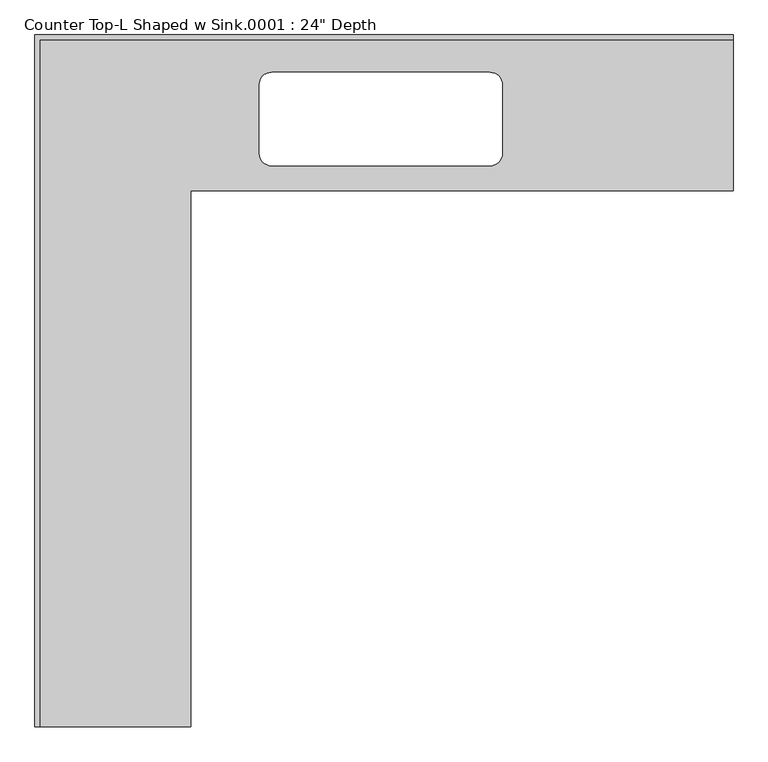
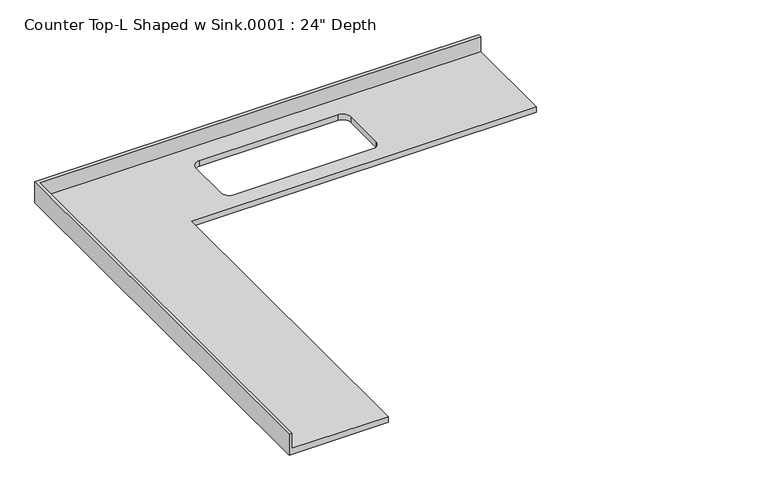
"""IFC4 building model written with IfcOpenShell, lengths in millimetres: furniture geometry."""

from ifc_helpers import new_model, si_unit, frame, origin, place, context, project, spatial, polyline, circle_curve, source, transform, mapped, element, save
from ifc_brep_helpers import plane_surface, revolved_surface, advanced_brep


def furniture_ce44b9f3(model_context):
    return source(origin(), model_context, "Body", "AdvancedBrep", [
        advanced_brep(
        [(-565.4622951, -2819.4, 914.4), (-565.4622951, -635.0, 914.4), (1644.3377049, -635.0, 914.4), (1644.3377049, -19.05, 914.4), (-1181.4122951, -19.05, 914.4), (-1181.4122951, -2819.4, 914.4), (653.7377049, -152.4, 914.4), (704.5377049, -203.2, 914.4), (704.5377049, -482.6, 914.4), (653.7377049, -533.4, 914.4), (-235.2622951, -533.4, 914.4), (-286.0622951, -482.6, 914.4), (-286.0622951, -203.2, 914.4), (-235.2622951, -152.4, 914.4), (1644.3377049, 0.0, 876.3), (1644.3377049, -635.0, 876.3), (-565.4622951, -635.0, 876.3), (-565.4622951, -2819.4, 876.3), (-1200.4622951, -2819.4, 876.3), (-1200.4622951, 0.0, 876.3), (653.7377049, -152.4, 876.3), (-235.2622951, -152.4, 876.3), (-286.0622951, -203.2, 876.3), (-286.0622951, -482.6, 876.3), (-235.2622951, -533.4, 876.3), (653.7377049, -533.4, 876.3), (704.5377049, -482.6, 876.3), (704.5377049, -203.2, 876.3), (-1200.4622951, 0.0, 1016.0), (1644.3377049, 0.0, 1016.0), (-1200.4622951, -2819.4, 1016.0), (-1181.4122951, -2819.4, 1016.0), (1644.3377049, -19.05, 1016.0), (-1181.4122951, -19.05, 1016.0)],
        [
            (0, 1),
            (1, 2),
            (2, 3),
            (3, 4),
            (4, 5),
            (5, 0),
            (6, 7, circle_curve(frame((653.7377049, -203.2, 914.4), z_axis=(0.0, 0.0, -1.0), x_axis=(1.0, 0.0, 0.0)), 50.8)),
            (7, 8),
            (8, 9, circle_curve(frame((653.7377049, -482.6, 914.4), z_axis=(0.0, 0.0, -1.0), x_axis=(1.0, 0.0, 0.0)), 50.8)),
            (9, 10),
            (10, 11, circle_curve(frame((-235.2622951, -482.6, 914.4), z_axis=(0.0, 0.0, -1.0), x_axis=(1.0, 0.0, 0.0)), 50.8)),
            (11, 12),
            (12, 13, circle_curve(frame((-235.2622951, -203.2, 914.4), z_axis=(0.0, 0.0, -1.0), x_axis=(1.0, 0.0, 0.0)), 50.8)),
            (13, 6),
            (14, 15),
            (15, 16),
            (16, 17),
            (17, 18),
            (18, 19),
            (19, 14),
            (20, 21),
            (21, 22, circle_curve(frame((-235.2622951, -203.2, 876.3), z_axis=(0.0, 0.0, 1.0), x_axis=(1.0, 0.0, 0.0)), 50.8)),
            (22, 23),
            (23, 24, circle_curve(frame((-235.2622951, -482.6, 876.3), z_axis=(0.0, 0.0, 1.0), x_axis=(1.0, 0.0, 0.0)), 50.8)),
            (24, 25),
            (25, 26, circle_curve(frame((653.7377049, -482.6, 876.3), z_axis=(0.0, 0.0, 1.0), x_axis=(1.0, 0.0, 0.0)), 50.8)),
            (26, 27),
            (27, 20, circle_curve(frame((653.7377049, -203.2, 876.3), z_axis=(0.0, 0.0, 1.0), x_axis=(1.0, 0.0, 0.0)), 50.8)),
            (19, 28),
            (28, 29),
            (29, 14),
            (18, 30),
            (30, 28),
            (17, 0),
            (5, 31),
            (31, 30),
            (16, 1),
            (15, 2),
            (29, 32),
            (32, 3),
            (6, 20),
            (27, 7),
            (26, 8),
            (25, 9),
            (24, 10),
            (23, 11),
            (22, 12),
            (21, 13),
            (31, 33),
            (33, 32),
            (33, 4),
        ],
        [
            plane_surface(frame((-1200.4622951, 0.0, 914.4), z_axis=(0.0, 0.0, 1.0), x_axis=(-1.0, 0.0, 0.0))),
            plane_surface(frame((-1200.4622951, 0.0, 876.3), z_axis=(0.0, 0.0, -1.0), x_axis=(1.0, 0.0, 0.0))),
            plane_surface(frame((1644.3377049, 0.0, 914.4), z_axis=(0.0, 1.0, 0.0), x_axis=(0.0, 0.0, -1.0))),
            plane_surface(frame((-1200.4622951, 0.0, 914.4), z_axis=(-1.0, 0.0, 0.0), x_axis=(0.0, 0.0, -1.0))),
            plane_surface(frame((-1200.4622951, -2819.4, 914.4), z_axis=(0.0, -1.0, 0.0), x_axis=(0.0, 0.0, -1.0))),
            plane_surface(frame((-565.4622951, -2819.4, 914.4), z_axis=(1.0, 0.0, 0.0), x_axis=(0.0, 0.0, -1.0))),
            plane_surface(frame((-565.4622951, -635.0, 914.4), z_axis=(0.0, -1.0, 0.0), x_axis=(0.0, 0.0, -1.0))),
            plane_surface(frame((1644.3377049, -635.0, 914.4), z_axis=(1.0, 0.0, 0.0), x_axis=(0.0, 0.0, -1.0))),
            revolved_surface(polyline([(704.5377049, -203.2, 876.3), (704.5377049, -203.2, 914.4)]), (653.7377049, -203.2, 0.0), (0.0, 0.0, -1.0)),
            plane_surface(frame((704.5377049, -203.2, 914.4), z_axis=(-1.0, 0.0, 0.0), x_axis=(0.0, 0.0, -1.0))),
            revolved_surface(polyline([(704.5377049, -482.6, 876.3), (704.5377049, -482.6, 914.4)]), (653.7377049, -482.6, 0.0), (0.0, 0.0, -1.0)),
            plane_surface(frame((653.7377049, -533.4, 914.4), z_axis=(0.0, 1.0, 0.0), x_axis=(0.0, 0.0, -1.0))),
            revolved_surface(polyline([(-184.4622951, -482.6, 876.3), (-184.4622951, -482.6, 914.4)]), (-235.2622951, -482.6, 0.0), (0.0, 0.0, -1.0)),
            plane_surface(frame((-286.0622951, -482.6, 914.4), z_axis=(1.0, 0.0, 0.0), x_axis=(0.0, 0.0, -1.0))),
            revolved_surface(polyline([(-184.4622951, -203.2, 876.3), (-184.4622951, -203.2, 914.4)]), (-235.2622951, -203.2, 0.0), (0.0, 0.0, -1.0)),
            plane_surface(frame((-235.2622951, -152.4, 914.4), z_axis=(0.0, -1.0, 0.0), x_axis=(0.0, 0.0, -1.0))),
            plane_surface(frame((-1200.4622951, 0.0, 1016.0), z_axis=(0.0, 0.0, 1.0), x_axis=(0.0, -1.0, 0.0))),
            plane_surface(frame((-1200.4622951, -19.05, 1016.0), z_axis=(0.0, -1.0, 0.0), x_axis=(0.0, 0.0, -1.0))),
            plane_surface(frame((-1181.4122951, -2819.4, 1016.0), z_axis=(1.0, 0.0, 0.0), x_axis=(0.0, 0.0, -1.0))),
        ],
        [
            (0, [[1, 2, 3, 4, 5, 6], [7, 8, 9, 10, 11, 12, 13, 14]]),
            (1, [[15, 16, 17, 18, 19, 20], [21, 22, 23, 24, 25, 26, 27, 28]]),
            (2, [[-20, 29, 30, 31]]),
            (3, [[-19, 32, 33, -29]]),
            (4, [[-32, -18, 34, -6, 35, 36]]),
            (5, [[-1, -34, -17, 37]]),
            (6, [[-2, -37, -16, 38]]),
            (7, [[-15, -31, 39, 40, -3, -38]]),
            (8, [[-7, 41, -28, 42]]),
            (9, [[-8, -42, -27, 43]]),
            (10, [[-9, -43, -26, 44]]),
            (11, [[-10, -44, -25, 45]]),
            (12, [[-11, -45, -24, 46]]),
            (13, [[-12, -46, -23, 47]]),
            (14, [[-13, -47, -22, 48]]),
            (15, [[-14, -48, -21, -41]]),
            (16, [[-33, -36, 49, 50, -39, -30]]),
            (17, [[-40, -50, 51, -4]]),
            (18, [[-49, -35, -5, -51]]),
        ],
    ),
    ])


if __name__ == "__main__":
    model = new_model("IFC4")
    model_context = context("Model", 3, world=origin())
    ifc_project = project(units=[si_unit("LENGTHUNIT", "METRE", prefix="MILLI")], contexts=[model_context])
    site = spatial("IfcSite", under=ifc_project)
    building = spatial("IfcBuilding", under=site)
    placement = place(None, origin())
    furniture_shape = furniture_ce44b9f3(model_context)
    element("IfcFurniture", 1, ObjectType="Counter Top-L Shaped w Sink.0001 : 24\" Depth", at=placement, inside=building, context=model_context, shape_type="MappedRepresentation", body=[
        mapped(furniture_shape, transform((0.0, 0.0, 0.0), x_axis=(1.0, 0.0, 0.0), y_axis=(0.0, 1.0, 0.0), z_axis=(0.0, 0.0, 1.0))),
    ])
    save(model, "model.ifc")

# Revit data of these elements
# Type "Counter Top-L Shaped w Sink.0001 : 24\" Depth"
#   Assembly Code = "C1030400"
#   Counter Thickness = 0' - 1 1/2"
#   Depth = 2' - 1"
#   Height = 3' - 0"
#   Length - Leg 1 [instance default] = 8' - 0"
#   Length - Leg 2 [instance default] = 6' - 0"
#   Sink Location [instance default] = 3' - 0"
#   Sink Location To Wall [instance default] = 0' - 6"
#   Sink Opening Depth [instance default] = 1' - 3"
#   Sink Opening Width [instance default] = 3' - 3"
#   Counter Top Material = none
#   Default Elevation = 0
# Element 1 (IfcFurniture, "Counter Top-L Shaped w Sink.0001 : 24\" Depth")
#   Length - Leg 1 = 9' - 4"
#   Length - Leg 2 = 9' - 3"
#   Materials on its faces: "Counter Top"
# Materials
#   "Counter Top": class "Wood", colour RGB 226 177 128, transparency 0
